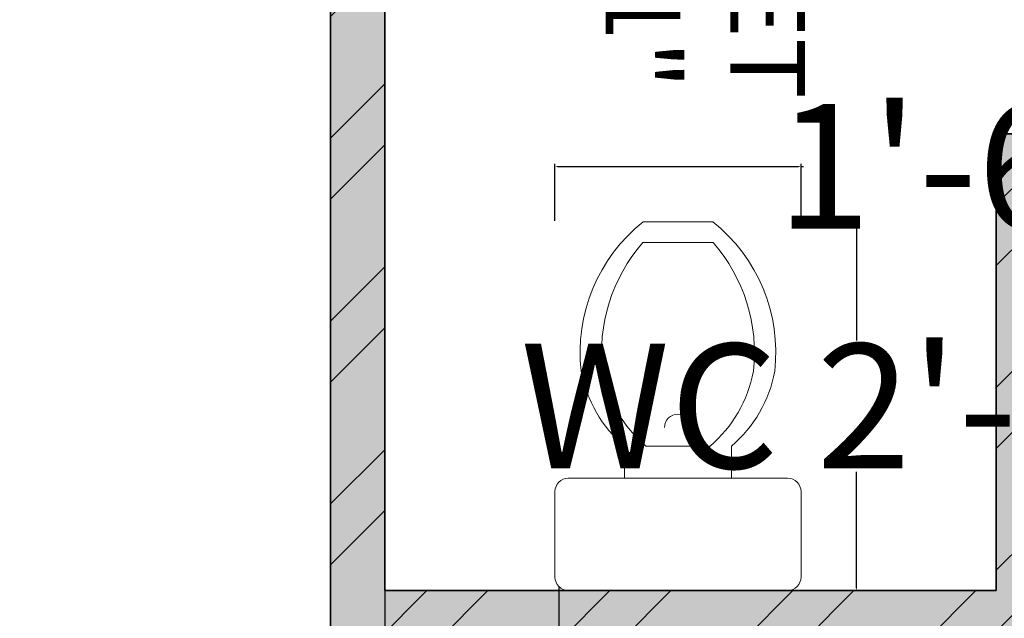
# Model space of a CAD drawing. Units: inches. Extents: x 1086 to 1540, y 3343 to 3848.
# Tile 4 of 8: x 1350 to 1422, y 3547 to 3591. Entities that reach past the tile are written whole.
import ezdxf

# ---------------------------------------------------------------- set-up
doc = ezdxf.new("R2010")
doc.units = ezdxf.units.IN
for name, color, linetype, lineweight in [('A-ANNO-DIMS', 2, 'Continuous', 13), ('A-AREA-IDEN', 7, 'Continuous', 18), ('A-FLOR-FIXT', 9, 'Continuous', 18), ('A-WALL-PATT', 252, 'Continuous', 9), ('WALL', 7, 'Continuous', 35)]:
    doc.layers.add(name, color=color, linetype=linetype, lineweight=lineweight)
doc.styles.get("Standard").update_dxf_attribs({"font": 'arial.ttf'})
doc.dimstyles.get("Standard").update_dxf_attribs({"dimtxt": 9.18, "dimasz": 0.18, "dimexe": 0.18, "dimexo": 0.0625, "dimgap": 0.09, "dimtad": 0, "dimtih": 1, "dimtoh": 1, "dimdec": 1, "dimzin": 0, "dimdsep": 46, "dimlunit": 3, "dimtxsty": 'Standard', "dimcen": 0.09, "dimadec": 0, "dimazin": 0, "dimtfac": 1, "dimtdec": 1, "dimtofl": 0, "dimtmove": 0, "dimatfit": 3, "dimfxl": 1, "dimtolj": 1, "dimtzin": 0, "dimarcsym": 0})

# ---------------------------------------------------------------- blocks, each defined once
blk = doc.blocks.new('A$C2AC94788')
for p, q in [((0.0250000842625013, 0.6899999873276103), (0.4350000842623559, 0.6899999873276103)), ((8.42619556e-08, 0.5049999873299384), (8.42619556e-08, 0.664999987326155)), ((0.4600000842619921, 0.664999987326155), (0.4600000842619921, 0.5049999873299384)), ((0.4350000842623559, 0.4799999873284833), (0.0250000842625013, 0.4799999873284833)), ((0.1300000842620648, 0.4799999873284833), (0.1300000842620648, 0.4199999873308116)), ((0.3300000842618829, 0.4199999873308116), (0.3300000842618829, 0.4799999873284833)), ((0.1700000842620284, 0.4199999873308116), (0.2900000842619192, 0.4199999873308116)), ((0.1640625266463758, 0.0391832446184708), (0.2959376418775719, 0.0391832446184708)), ((0.2290625266468851, 0.0391832446184708), (0.2300046331329213, 0.0391832446184708)), ((0.2309376418770626, 0.0391832446184708), (0.2299955353910263, 0.0391832446184708)), ((0.1650000842619192, -1.26747182e-08), (0.2950000842620284, -1.26747182e-08))]:
    blk.add_line(p, q)
for centre, radius, start, end in [((0.0250000842625013, 0.664999987326155), 0.025, 90, 180), ((0.4350000842623559, 0.664999987326155), 0.025, 0, 90), ((0.0250000842625013, 0.5049999873299384), 0.025, 180, 270), ((0.4350000842623559, 0.5049999873299384), 0.025, 270, 0), ((0.2874442183401697, 0.2355819240110577), 0.2424843859558644, 130.488541879527, 169.445013547103), ((0.3274442183401334, 0.2355819240110577), 0.2424843859558644, 130.488541879527, 169.445013547103), ((0.1325559501838143, 0.2355819240110577), 0.2424843859558745, 10.55498645289699, 49.51145812047296), ((0.1725559501837779, 0.2355819240110577), 0.2424843859558745, 10.55498645289699, 49.51145812047296), ((0.2300000842624286, 0.3849999873273191), 0.025, 180, 0), ((0.3600593119572294, 0.2447691737834247), 0.3129857136460789, 173.5368801771597, 231.4482773914608), ((0.4000593119571932, 0.2447691737834248), 0.3129857136460972, 173.5368801771598, 221.0603827222079), ((0.0999408565667182, 0.2447691737834248), 0.3129857136460789, 308.5517226085392, 6.463119822840183), ((0.0599408565667545, 0.2447691737834248), 0.3129857136460896, 318.9396172777922, 6.463119822840183)]:
    blk.add_arc(centre, radius, start, end)
blk = doc.blocks.new('*D35')
at = {"layer": 'A-ANNO-DIMS', "color": 0, "lineweight": -2, "transparency": 16777216}
for p, q in [((1407.435838009893, 3575.739529833988), (1411.628650509907, 3575.739529833988)), ((1411.448650509907, 3575.559529833988), (1411.448650509907, 3566.99483423367)), ((1411.448650509907, 3548.750779833896), (1411.448650509907, 3557.315475434215)), ((1407.435838009893, 3548.570779833897), (1411.628650509907, 3548.570779833897))]:
    blk.add_line(p, q, dxfattribs=at)
at = {"layer": 'A-ANNO-DIMS', "color": 0, "transparency": 16777216}
for points in [[(1411.418650509907, 3575.559529833988), (1411.478650509907, 3575.559529833988), (1411.448650509907, 3575.739529833988)], [(1411.418650509907, 3548.750779833896), (1411.478650509907, 3548.750779833896), (1411.448650509907, 3548.570779833897)]]:
    blk.add_solid(points, dxfattribs=at)
at = {"layer": 'Defpoints', "color": 0, "transparency": 16777216}
for p in [(1407.373338009892, 3575.739529833988), (1407.373338009892, 3548.570779833897), (1411.448650509907, 3548.570779833897)]:
    blk.add_point(p, dxfattribs=at)
at = {"layer": 'A-ANNO-DIMS', "color": 0, "transparency": 16777216, "insert": (1411.448650509908, 3562.155154833941), "char_height": 9.18, "attachment_point": 5}
blk.add_mtext('\\A1;WC 2\'-3"', dxfattribs=at)
blk = doc.blocks.new('*D36')
at = {"layer": 'A-ANNO-DIMS', "color": 0, "lineweight": -2, "transparency": 16777216}
for p, q in [((1389.260838009876, 3575.802029833987), (1389.260838009876, 3579.994842334)), ((1389.440838009876, 3579.814842334001), (1407.193338009892, 3579.814842334001)), ((1407.373338009892, 3575.802029833987), (1407.373338009892, 3579.994842334)), ((1407.373338009892, 3579.814842334001), (1407.553338009892, 3579.814842334001))]:
    blk.add_line(p, q, dxfattribs=at)
at = {"layer": 'A-ANNO-DIMS', "color": 0, "transparency": 16777216}
for points in [[(1389.440838009876, 3579.844842334), (1389.440838009876, 3579.784842334), (1389.260838009876, 3579.814842334001)], [(1407.193338009892, 3579.844842334), (1407.193338009892, 3579.784842334), (1407.373338009892, 3579.814842334001)]]:
    blk.add_solid(points, dxfattribs=at)
at = {"layer": 'Defpoints', "color": 0, "transparency": 16777216}
for p in [(1407.373338009892, 3579.814842334001), (1389.260838009876, 3575.739529833987), (1407.373338009892, 3575.739529833987)]:
    blk.add_point(p, dxfattribs=at)
at = {"layer": 'A-ANNO-DIMS', "color": 0, "transparency": 16777216, "insert": (1419.41264906037, 3579.814842334001), "char_height": 9.18, "attachment_point": 5}
blk.add_mtext('\\A1;1\'-6"', dxfattribs=at)
blk = doc.blocks.new('*D66')
at = {"layer": 'A-ANNO-DIMS', "color": 0, "lineweight": -2, "transparency": 16777216}
for p, q in [((1389.549155, 3548.796597), (1389.549155, 3356.390778)), ((1376.740448, 3548.50828), (1376.740448, 3356.390778)), ((1376.920448, 3356.570778), (1389.369155, 3356.570778)), ((1389.549155, 3356.570778), (1389.729155, 3356.570778))]:
    blk.add_line(p, q, dxfattribs=at)
at = {"layer": 'A-ANNO-DIMS', "color": 0, "transparency": 16777216}
for points in [[(1376.920448, 3356.600778), (1376.920448, 3356.540777999999), (1376.740448, 3356.570778)], [(1389.369155, 3356.600778), (1389.369155, 3356.540777999999), (1389.549155, 3356.570778)]]:
    blk.add_solid(points, dxfattribs=at)
at = {"layer": 'Defpoints', "color": 0, "transparency": 16777216}
for p in [(1376.740448, 3548.57078), (1389.549155, 3548.859097000001), (1389.549155, 3356.570778)]:
    blk.add_point(p, dxfattribs=at)
at = {"layer": 'A-ANNO-DIMS', "color": 0, "transparency": 16777216, "insert": (1401.588466050477, 3356.570778), "char_height": 9.18, "attachment_point": 5}
blk.add_mtext('\\A1;1\'-1"', dxfattribs=at)

msp = doc.modelspace()

# ---------------------------------------------------------------- hatches: boundary and pattern name
at = {"layer": 'A-WALL-PATT'}
h = msp.add_hatch(dxfattribs=at)
h.set_pattern_fill('ANSI32', color=256)
h.set_pattern_definition([(45, (0, 0), (-6.735192090801865, 6.735192090801866), []), (45, (4.49013, 0), (-6.735192090801865, 6.735192090801866), [])])
h.paths.add_polyline_path([(1234.550507268797, 3811.570780184086), (1234.550506085547, 3811.570780184086), (1194.74044790643, 3811.570780204329), (1194.74044790643, 3622.570780204329), (1203.74044790643, 3622.570780204329), (1203.74044790643, 3634.57078020433), (1218.334481095046, 3634.57078020433), (1218.334481095046, 3638.570780204329), (1203.74044790643, 3638.570780204329), (1203.74044790643, 3802.570780204329), (1234.550507268797, 3802.570780204328)])
h.paths.add_polyline_path([(1371.059017457095, 3811.570780184086), (1371.059016273845, 3811.570780184086), (1282.550507268797, 3811.570780204329), (1282.550507268797, 3802.570780204328), (1331.74044790643, 3802.570780204329), (1331.74044790643, 3634.57078020433), (1335.740443663098, 3634.570780204329), (1335.740443663098, 3639.570779622127), (1335.74044790643, 3802.570780204329), (1371.059017457095, 3802.570780204329)])
h.paths.add_polyline_path([(1470.74044790643, 3811.570780204329), (1419.059017457095, 3811.570780204329), (1419.059017457094, 3802.570780204329), (1461.74044790643, 3802.570780204329), (1461.74044790643, 3638.570780204329), (1461.74044790643, 3548.570780204335), (1425.74044790643, 3548.570780204334), (1425.74044790643, 3582.213777424251), (1421.74044790643, 3582.213777424251), (1421.74044790643, 3548.570780204334), (1376.74044790643, 3548.570780204333), (1376.74044790643, 3602.570780204329), (1373.714630900908, 3602.570780204329), (1372.74044790643, 3602.570780204329), (1372.74044790643, 3544.570780204329), (1461.74044790643, 3544.570780204332), (1461.74044790643, 3379.57078020433), (1470.74044790643, 3379.570780204329)])
h.paths.add_polyline_path([(1203.74044790643, 3582.570780204329), (1295.74044790643, 3582.57078020433), (1295.74044790643, 3586.57078020433), (1203.74044790643, 3586.570780204329), (1203.74044790643, 3598.570780204329), (1194.74044790643, 3598.570780204329), (1194.74044790643, 3379.570780204329), (1326.74044790643, 3379.570780204329), (1326.74044790643, 3388.570780204329), (1322.74044790643, 3388.570780204329), (1203.74044790643, 3388.570780204329), (1203.74044790643, 3451.570780204329), (1234.74044790643, 3451.570780204329), (1234.740447906429, 3455.570780204329), (1203.74044790643, 3455.570780204329), (1203.74044790643, 3479.570780204329), (1203.74044790643, 3544.570780204329), (1227.74044790643, 3544.570780204329), (1253.74044790643, 3544.570780204329), (1253.74044790643, 3548.570780204329), (1203.74044790643, 3548.570780204329)])
h.paths.add_polyline_path([(1461.74044790643, 3638.570780204329), (1371.74044790643, 3638.570780204329), (1371.74044790643, 3634.570780204329), (1372.74044790643, 3634.57078020433), (1372.74044790643, 3632.570780204328), (1376.74044790643, 3632.570780204328), (1376.74044790643, 3634.570780204329), (1421.74044790643, 3634.57078020433), (1421.74044790643, 3606.21377742425), (1425.74044790643, 3606.213777424251), (1425.74044790643, 3634.57078020433), (1461.74044790643, 3634.57078020433)])
h.paths.add_polyline_path([(1295.740445944246, 3638.570780204329), (1266.334481095045, 3638.570780204329), (1266.334481095045, 3634.57078020433), (1292.74044790643, 3634.57078020433), (1295.740445944246, 3634.57078020433)])
h.paths.add_polyline_path([(1322.74044790643, 3548.570780204332), (1318.74044790643, 3548.570780204331), (1318.74044790643, 3455.570780204329), (1282.74044790643, 3455.570780204329), (1282.74044790643, 3451.57078020433), (1318.74044790643, 3451.57078020433), (1318.74044790643, 3420.07078020433), (1322.74044790643, 3420.07078020433)], flags=17)
at = {"layer": 'A-WALL-PATT', "transparency": 33554559}
h = msp.add_hatch(color=256, dxfattribs=at)
h.dxf.hatch_style = 1
h.paths.add_polyline_path([(1234.550507268797, 3811.570780184086), (1234.550506085547, 3811.570780184086), (1194.74044790643, 3811.570780204329), (1194.74044790643, 3622.570780204329), (1203.74044790643, 3622.570780204329), (1203.74044790643, 3634.57078020433), (1218.334481095046, 3634.57078020433), (1218.334481095046, 3638.570780204329), (1203.74044790643, 3638.570780204329), (1203.74044790643, 3802.570780204329), (1234.550507268797, 3802.570780204328)])
h.paths.add_polyline_path([(1371.059017457095, 3811.570780184086), (1371.059016273845, 3811.570780184086), (1282.550507268797, 3811.570780204329), (1282.550507268797, 3802.570780204328), (1331.74044790643, 3802.570780204329), (1331.74044790643, 3634.57078020433), (1335.740443663098, 3634.570780204329), (1335.740443663098, 3639.570779622127), (1335.74044790643, 3802.570780204329), (1371.059017457095, 3802.570780204329)])
h.paths.add_polyline_path([(1470.74044790643, 3811.570780204329), (1419.059017457095, 3811.570780204329), (1419.059017457094, 3802.570780204329), (1461.74044790643, 3802.570780204329), (1461.74044790643, 3638.570780204329), (1461.74044790643, 3548.570780204335), (1425.74044790643, 3548.570780204334), (1425.74044790643, 3582.213777424251), (1421.74044790643, 3582.213777424251), (1421.74044790643, 3548.570780204334), (1376.74044790643, 3548.570780204333), (1376.74044790643, 3602.570780204328), (1372.74044790643, 3602.570780204329), (1372.74044790643, 3544.570780204329), (1461.74044790643, 3544.570780204332), (1461.74044790643, 3379.57078020433), (1470.74044790643, 3379.570780204329)])
h.paths.add_polyline_path([(1203.74044790643, 3544.570780204329), (1227.74044790643, 3544.570780204329), (1253.74044790643, 3544.570780204329), (1253.74044790643, 3548.570780204329), (1203.74044790643, 3548.570780204329), (1203.74044790643, 3582.570780204329), (1295.74044790643, 3582.57078020433), (1295.74044790643, 3586.57078020433), (1203.74044790643, 3586.570780204329), (1203.74044790643, 3598.570780204329), (1194.74044790643, 3598.570780204329), (1194.74044790643, 3379.570780204329), (1326.74044790643, 3379.570780204329), (1326.74044790643, 3388.570780204329), (1322.74044790643, 3388.570780204329), (1203.74044790643, 3388.570780204329), (1203.74044790643, 3451.570780204329), (1234.74044790643, 3451.570780204329), (1234.740447906429, 3455.570780204329), (1203.74044790643, 3455.570780204329)])
h.paths.add_polyline_path([(1413.74044790643, 3388.570780184088), (1413.740446723181, 3388.570780184088), (1374.74044790643, 3388.570780204329), (1374.74044790643, 3383.179800700248), (1374.74045402255, 3383.179800700248), (1374.740454022761, 3379.570780204329), (1413.74044790643, 3379.57078020433)], flags=17)
h.paths.add_polyline_path([(1322.74044790643, 3548.570780204332), (1318.74044790643, 3548.570780204331), (1318.74044790643, 3455.570780204329), (1282.74044790643, 3455.570780204329), (1282.74044790643, 3451.57078020433), (1318.74044790643, 3451.57078020433), (1318.74044790643, 3420.07078020433), (1322.74044790643, 3420.07078020433)], flags=17)
h.paths.add_polyline_path([(1295.740445944246, 3638.570780204329), (1266.334481095045, 3638.570780204329), (1266.334481095045, 3634.57078020433), (1292.74044790643, 3634.57078020433), (1295.740445944246, 3634.57078020433)])
h.paths.add_polyline_path([(1461.74044790643, 3638.570780204329), (1371.74044790643, 3638.570780204329), (1371.74044790643, 3634.570780204329), (1372.74044790643, 3634.57078020433), (1372.74044790643, 3632.570780204328), (1376.74044790643, 3632.570780204328), (1376.74044790643, 3634.570780204329), (1421.74044790643, 3634.57078020433), (1421.74044790643, 3606.21377742425), (1425.74044790643, 3606.213777424251), (1425.74044790643, 3634.57078020433), (1461.74044790643, 3634.57078020433)])

# ---------------------------------------------------------------- linework, layer by layer
at = {"layer": 'WALL'}
for p, q in [((1372.74044790643, 3602.570780204329), (1372.74044790643, 3544.57078020433)), ((1376.74044790643, 3602.57078020433), (1376.74044790643, 3548.570780204333)), ((1425.74044790643, 3582.213777424251), (1421.74044790643, 3582.213777424251)), ((1421.74044790643, 3582.213777424251), (1421.74044790643, 3548.570780204334)), ((1376.74044790643, 3548.570780204333), (1421.74044790643, 3548.570780204334))]:
    msp.add_line(p, q, dxfattribs=at)

# ---------------------------------------------------------------- block references
at = {"layer": 'A-FLOR-FIXT', "xscale": -39.375, "yscale": 39.375, "zscale": 39.375, "rotation": 180}
msp.add_blockref('A$C2AC94788', (1389.260834692062, 3575.739529334919), dxfattribs=at)

# ---------------------------------------------------------------- texts
at = {"layer": 'A-AREA-IDEN', "insert": (1407.667173371051, 3610.037077309889), "char_height": 8, "attachment_point": 1, "rotation": 270}
msp.add_mtext_dynamic_manual_height_columns('{\\H0.6875x;TOILET\\P7\'X4\'1"} ', width=58.98782469678554, gutter_width=0, heights=[37.043222458365], dxfattribs=at)

# ---------------------------------------------------------------- dimensions: what is measured, and where the dimension line sits
at = {"layer": 'A-ANNO-DIMS'}
for base, p1, p2, picture, middle in [((1407.373338009892, 3579.814842334001), (1389.260838009876, 3575.739529833987), (1407.373338009892, 3575.739529833987), '*D36', (1419.41264906037, 3579.814842334001)), ((1389.549155, 3356.570778), (1376.740448, 3548.57078), (1389.549155, 3548.859097000001), '*D66', (1401.588466050477, 3356.570778))]:
    dim = msp.add_linear_dim(base=base, p1=p1, p2=p2, dimstyle='Standard', override={"dimdec": 1, "dimlfac": 1, "dimrnd": 0, "dimzin": 1, "dimdsep": 46, "dimlunit": 4, "dimfrac": 2}, dxfattribs=at)
    dim.commit()
    dim.dimension.update_dxf_attribs({"geometry": picture, "text_midpoint": middle})
dim = msp.add_linear_dim(base=(1411.448650509907, 3548.570779833897), p1=(1407.373338009892, 3575.739529833987), p2=(1407.373338009892, 3548.570779833895), angle=270, text='WC <>', dimstyle='Standard', override={"dimdec": 1, "dimlfac": 1, "dimrnd": 0, "dimzin": 1, "dimdsep": 46, "dimlunit": 4, "dimfrac": 2}, dxfattribs=at)
dim.commit()
dim.dimension.update_dxf_attribs({"geometry": '*D35', "text_midpoint": (1411.448650509908, 3562.155154833941)})

doc.saveas('drawing.dxf')
